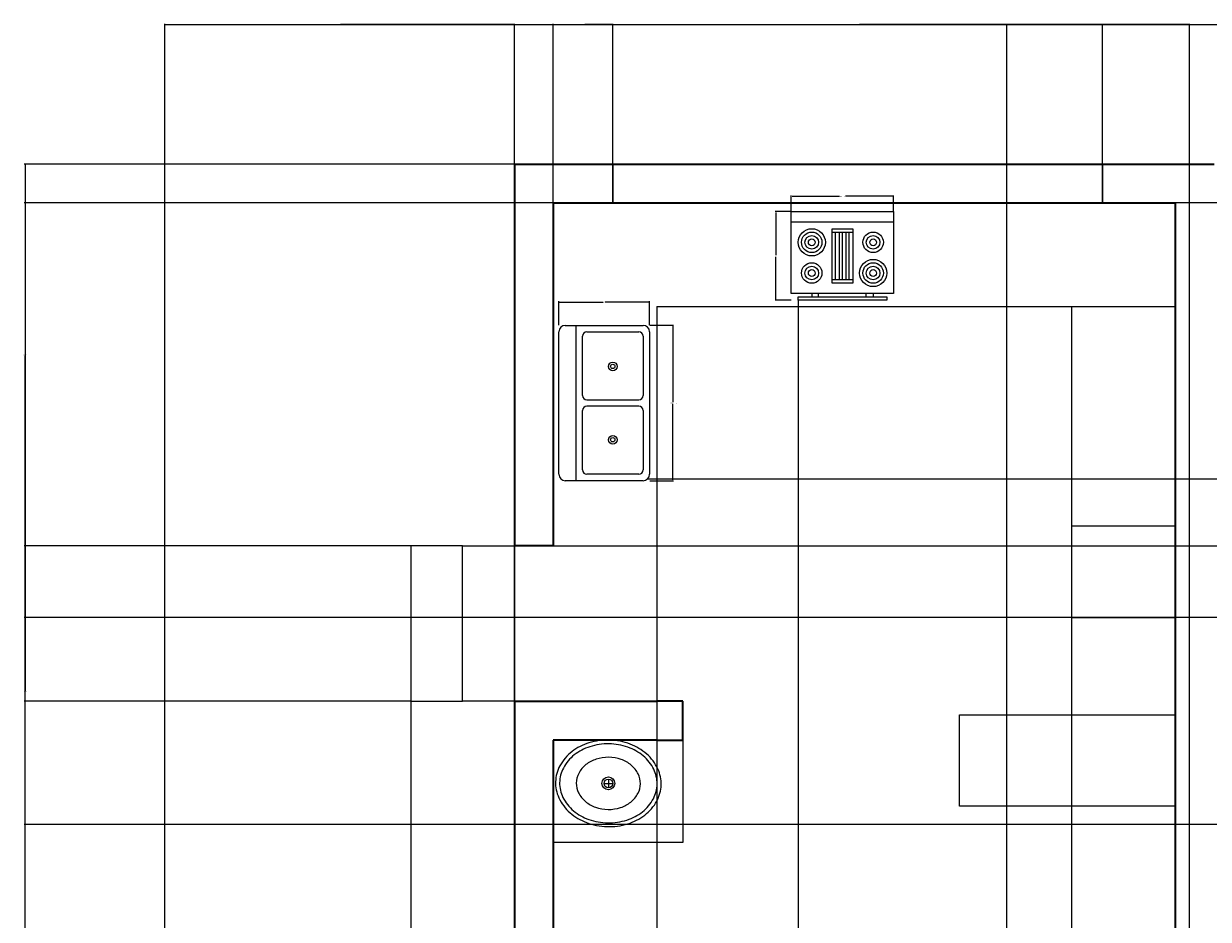
# Model space of a CAD drawing. Units: inches. Extents: x 1159 to 1869, y 2212 to 2738.
# Tile 2 of 5: x 1159 to 1433, y 2531 to 2738. Entities that reach past the tile are written whole.
import ezdxf

# ---------------------------------------------------------------- set-up
doc = ezdxf.new("R2010")
doc.units = ezdxf.units.IN
for name, color, linetype, lineweight in [('A-ANNO-DIMS', 2, 'Continuous', 18), ('A-EQPM', 8, 'Continuous', 18), ('A-FLOR-CASE', 30, 'Continuous', 18), ('A-FLOR-FIXT', 9, 'Continuous', 18), ('A-FLOR-STRS', 7, 'Continuous', 25), ('A-GLAZ', 4, 'Continuous', 18), ('A-WALL', 7, 'Continuous', 35)]:
    doc.layers.add(name, color=color, linetype=linetype, lineweight=lineweight)
doc.styles.get("Standard").update_dxf_attribs({"font": 'arial.ttf'})
doc.dimstyles.get("Standard").update_dxf_attribs({"dimtxt": 0.18, "dimasz": 0.18, "dimexe": 0.18, "dimexo": 0.0625, "dimgap": 0.09, "dimtad": 0, "dimtih": 1, "dimtoh": 1, "dimdec": 4, "dimzin": 0, "dimdsep": 46, "dimtxsty": 'Standard', "dimcen": 0.09, "dimadec": 0, "dimazin": 0, "dimtfac": 1, "dimtdec": 4, "dimtofl": 0, "dimtmove": 0, "dimatfit": 3, "dimfxl": 1, "dimtolj": 1, "dimtzin": 0, "dimarcsym": 0})

# ---------------------------------------------------------------- blocks, each defined once
blk = doc.blocks.new('Sink - Oval top')
for p, q in [((-1, 0), (1, 0)), ((0, 1), (0, -1))]:
    blk.add_line(p, q)
for points in [[(-12.23, 0.39, 0.117634), (-11.46, -3.36, 0.104469), (-8.88, -6.8, 0.090016), (-5.08, -9.07, 0.08192), (-0.32, -10.02, 0.08192), (4.49, -9.38, 0.090016), (8.42, -7.36, 0.104469), (11.22, -4.09, 0.117634), (12.23, -0.39, 0.117634), (11.46, 3.36, 0.104469), (8.88, 6.8, 0.090016), (5.08, 9.07, 0.08192), (0.32, 10.02, 0.08192), (-4.49, 9.38, 0.090016), (-8.42, 7.36, 0.104469), (-11.22, 4.09, 0.117634)], [(-11.29, 0.16, 0.118622), (-10.52, -3.25, 0.104678), (-8.07, -6.36, 0.089562), (-4.54, -8.37, 0.081185), (-0.13, -9.15, 0.081185), (4.3, -8.49, 0.089562), (7.89, -6.58, 0.104678), (10.42, -3.55, 0.118622), (11.29, -0.16, 0.118622), (10.52, 3.25, 0.104678), (8.07, 6.36, 0.089562), (4.54, 8.37, 0.081185), (0.13, 9.15, 0.081185), (-4.3, 8.49, 0.089562), (-7.89, 6.58, 0.104678), (-10.42, 3.55, 0.118622)], [(-7.42, 0.08, 0.118283), (-6.91, -2.17, 0.104607), (-5.29, -4.21, 0.089718), (-2.97, -5.53, 0.081436), (-0.07, -6.04, 0.081436), (2.84, -5.59, 0.089718), (5.2, -4.33, 0.104607), (6.86, -2.32, 0.118283), (7.42, -0.08, 0.118283), (6.91, 2.17, 0.104607), (5.29, 4.21, 0.089718), (2.97, 5.53, 0.081436), (0.07, 6.04, 0.081436), (-2.84, 5.59, 0.089718), (-5.2, 4.33, 0.104607), (-6.86, 2.32, 0.118283)]]:
    blk.add_lwpolyline(points, format="xyb", close=True)
for radius in [1.5, 1]:
    blk.add_circle((0, 0), radius)
blk = doc.blocks.new('Sink-double - 36 in top')
for p, q in [((-18, -4), (18, -4)), ((-0.75, -18.5), (-0.75, -6.5)), ((0.75, -6.5), (0.75, -18.5))]:
    blk.add_line(p, q)
for points in [[(-16.5, 0), (16.5, 0)], [(-18, -19.5), (-18, -1.5)], [(18, -1.5), (18, -19.5)], [(-16.5, -18.5), (-16.5, -6.5)], [(-15.5, -5.5), (-1.75, -5.5)], [(1.75, -5.5), (15.5, -5.5)], [(16.5, -6.5), (16.5, -18.5)], [(16.5, -21), (-16.5, -21)], [(-1.75, -19.5), (-15.5, -19.5)], [(15.5, -19.5), (1.75, -19.5)]]:
    blk.add_lwpolyline(points)
for centre, radius in [((-8.5, -12.5), 1), ((-8.5, -12.5), 0.5), ((8.5, -12.5), 1), ((8.5, -12.5), 0.5)]:
    blk.add_circle(centre, radius)
for centre, radius, start, end in [((-16.5, -1.5), 1.5, 90, 180), ((16.5, -1.5), 1.5, 0, 90), ((-15.5, -6.5), 1, 90, 180), ((-1.75, -6.5), 1, 0, 90), ((1.75, -6.5), 1, 90, 180), ((15.5, -6.5), 1, 0, 90), ((-15.5, -18.5), 1, 180, 270), ((-1.75, -18.5), 1, 270, 0), ((1.75, -18.5), 1, 180, 270), ((15.5, -18.5), 1, 270, 0), ((-16.5, -19.5), 1.5, 180, 270), ((16.5, -19.5), 1.5, 270, 0)]:
    blk.add_arc(centre, radius, start, end)
blk = doc.blocks.new('Range-Oven - 30 in top')
for p, q in [((0, -3), (30, -3)), ((12, -6), (18, -6)), ((13, -20), (13, -6)), ((14, -6), (14, -20)), ((15, -20), (15, -6)), ((16, -6), (16, -20)), ((17, -20), (17, -6)), ((18, -20), (12, -20)), ((6, -24), (6, -25)), ((8, -25), (8, -24)), ((22, -25), (22, -24)), ((24, -24), (24, -25))]:
    blk.add_line(p, q)
for points in [[(0, -24), (0, 0), (30, 0), (30, -24)], [(12, -21), (12, -5), (18, -5), (18, -21)], [(2, -26), (2, -25), (28, -25), (28, -26)]]:
    blk.add_lwpolyline(points, close=True)
for centre, radius in [((6, -9), 4), ((6, -9), 3), ((24, -9), 3), ((6, -9), 2), ((6, -9), 1), ((24, -9), 2), ((24, -9), 1), ((6, -18), 3), ((6, -18), 2), ((6, -18), 1), ((24, -18), 4), ((24, -18), 3), ((24, -18), 2), ((24, -18), 1)]:
    blk.add_circle(centre, radius)
blk = doc.blocks.new('*D16')
at = {"layer": 'A-ANNO-DIMS', "color": 0, "lineweight": -2, "transparency": 16777216}
for p, q in [((1303.74, 2668.28), (1309.26, 2668.28)), ((1309.08, 2668.1), (1309.08, 2650.46)), ((1309.08, 2632.46), (1309.08, 2650.09)), ((1303.74, 2632.28), (1309.26, 2632.28))]:
    blk.add_line(p, q, dxfattribs=at)
at = {"layer": 'A-ANNO-DIMS', "color": 0, "transparency": 16777216}
for points in [[(1309.05, 2668.1), (1309.11, 2668.1), (1309.08, 2668.28)], [(1309.05, 2632.46), (1309.11, 2632.46), (1309.08, 2632.28)]]:
    blk.add_solid(points, dxfattribs=at)
at = {"layer": 'Defpoints', "color": 0, "transparency": 16777216}
for p in [(1303.68, 2668.28), (1309.08, 2668.28), (1303.68, 2632.28)]:
    blk.add_point(p, dxfattribs=at)
at = {"layer": 'A-ANNO-DIMS', "color": 0, "transparency": 16777216, "insert": (1309.08, 2650.28), "char_height": 0.18, "attachment_point": 5}
blk.add_mtext('\\A1;DOUBLE SINK 36', dxfattribs=at)
blk = doc.blocks.new('*D17')
at = {"layer": 'A-ANNO-DIMS', "color": 0, "lineweight": -2, "transparency": 16777216}
for p, q in [((1282.68, 2668.34), (1282.68, 2673.86)), ((1282.86, 2673.68), (1292.97, 2673.68)), ((1303.5, 2673.68), (1293.38, 2673.68)), ((1303.68, 2668.34), (1303.68, 2673.86))]:
    blk.add_line(p, q, dxfattribs=at)
at = {"layer": 'A-ANNO-DIMS', "color": 0, "transparency": 16777216}
for points in [[(1282.86, 2673.71), (1282.86, 2673.65), (1282.68, 2673.68)], [(1303.5, 2673.71), (1303.5, 2673.65), (1303.68, 2673.68)]]:
    blk.add_solid(points, dxfattribs=at)
at = {"layer": 'Defpoints', "color": 0, "transparency": 16777216}
for p in [(1282.68, 2673.68), (1282.68, 2668.28), (1303.68, 2668.28)]:
    blk.add_point(p, dxfattribs=at)
at = {"layer": 'A-ANNO-DIMS', "color": 0, "transparency": 16777216, "insert": (1293.18, 2673.68), "char_height": 0.18, "attachment_point": 5}
blk.add_mtext('\\A1;21', dxfattribs=at)
blk = doc.blocks.new('*D18')
at = {"layer": 'A-ANNO-DIMS', "color": 0, "lineweight": -2, "transparency": 16777216}
for p, q in [((1336.51, 2694.68), (1336.51, 2698.35)), ((1336.69, 2698.17), (1347.66, 2698.17)), ((1360.02, 2698.17), (1349.05, 2698.17)), ((1360.2, 2694.68), (1360.2, 2698.35))]:
    blk.add_line(p, q, dxfattribs=at)
at = {"layer": 'A-ANNO-DIMS', "color": 0, "transparency": 16777216}
for points in [[(1336.69, 2698.2), (1336.69, 2698.14), (1336.51, 2698.17)], [(1360.02, 2698.2), (1360.02, 2698.14), (1360.2, 2698.17)]]:
    blk.add_solid(points, dxfattribs=at)
at = {"layer": 'Defpoints', "color": 0, "transparency": 16777216}
for p in [(1360.2, 2698.17), (1336.51, 2694.61), (1360.2, 2694.61)]:
    blk.add_point(p, dxfattribs=at)
at = {"layer": 'A-ANNO-DIMS', "color": 0, "transparency": 16777216, "insert": (1348.35, 2698.17), "char_height": 0.18, "attachment_point": 5}
blk.add_mtext('\\A1;RANGE 24', dxfattribs=at)
blk = doc.blocks.new('*D19')
at = {"layer": 'A-ANNO-DIMS', "color": 0, "lineweight": -2, "transparency": 16777216}
for p, q in [((1336.44, 2694.61), (1332.77, 2694.61)), ((1332.95, 2694.43), (1332.95, 2684.53)), ((1332.95, 2674.26), (1332.95, 2684.17)), ((1336.44, 2674.08), (1332.77, 2674.08))]:
    blk.add_line(p, q, dxfattribs=at)
at = {"layer": 'A-ANNO-DIMS', "color": 0, "transparency": 16777216}
for points in [[(1332.92, 2694.43), (1332.98, 2694.43), (1332.95, 2694.61)], [(1332.92, 2674.26), (1332.98, 2674.26), (1332.95, 2674.08)]]:
    blk.add_solid(points, dxfattribs=at)
at = {"layer": 'Defpoints', "color": 0, "transparency": 16777216}
for p in [(1332.95, 2694.61), (1336.51, 2694.61), (1336.51, 2674.08)]:
    blk.add_point(p, dxfattribs=at)
at = {"layer": 'A-ANNO-DIMS', "color": 0, "transparency": 16777216, "insert": (1332.95, 2684.35), "char_height": 0.18, "attachment_point": 5}
blk.add_mtext('\\A1;21', dxfattribs=at)
blk = doc.blocks.new('*D20')
at = {"layer": 'A-ANNO-DIMS', "color": 0, "lineweight": -2, "transparency": 16777216}
for p, q in [((1191.4, 2461.27), (1191.4, 2738.15)), ((1191.58, 2737.97), (1513.61, 2737.97)), ((1836.22, 2737.97), (1514.19, 2737.97)), ((1836.4, 2705.69), (1836.4, 2738.15))]:
    blk.add_line(p, q, dxfattribs=at)
at = {"layer": 'A-ANNO-DIMS', "color": 0, "transparency": 16777216}
for points in [[(1191.58, 2738), (1191.58, 2737.94), (1191.4, 2737.97)], [(1836.22, 2738), (1836.22, 2737.94), (1836.4, 2737.97)]]:
    blk.add_solid(points, dxfattribs=at)
at = {"layer": 'Defpoints', "color": 0, "transparency": 16777216}
for p in [(1836.4, 2737.97), (1836.4, 2705.63), (1191.4, 2461.21)]:
    blk.add_point(p, dxfattribs=at)
at = {"layer": 'A-ANNO-DIMS', "color": 0, "transparency": 16777216, "insert": (1513.9, 2737.97), "char_height": 0.18, "attachment_point": 5}
blk.add_mtext('\\A1;645', dxfattribs=at)
blk = doc.blocks.new('*D22')
at = {"layer": 'A-ANNO-DIMS', "color": 0, "lineweight": -2, "transparency": 16777216}
for p, q in [((1191.4, 2461.27), (1191.4, 2738.15)), ((1191.58, 2737.97), (1231.7, 2737.97)), ((1272.22, 2737.97), (1232.1, 2737.97)), ((1272.4, 2461.27), (1272.4, 2738.15))]:
    blk.add_line(p, q, dxfattribs=at)
at = {"layer": 'A-ANNO-DIMS', "color": 0, "transparency": 16777216}
for points in [[(1191.58, 2738), (1191.58, 2737.94), (1191.4, 2737.97)], [(1272.22, 2738), (1272.22, 2737.94), (1272.4, 2737.97)]]:
    blk.add_solid(points, dxfattribs=at)
at = {"layer": 'Defpoints', "color": 0, "transparency": 16777216}
for p in [(1272.4, 2737.97), (1191.4, 2461.21), (1272.4, 2461.21)]:
    blk.add_point(p, dxfattribs=at)
at = {"layer": 'A-ANNO-DIMS', "color": 0, "transparency": 16777216, "insert": (1231.9, 2737.97), "char_height": 0.18, "attachment_point": 5}
blk.add_mtext('\\A1;81', dxfattribs=at)
blk = doc.blocks.new('*D23')
at = {"layer": 'A-ANNO-DIMS', "color": 0, "lineweight": -2, "transparency": 16777216}
for p, q in [((1425.4, 2556.85), (1425.4, 2211.56)), ((1281.4, 2548.45), (1281.4, 2211.56)), ((1281.58, 2211.74), (1353.12, 2211.74)), ((1425.22, 2211.74), (1353.68, 2211.74))]:
    blk.add_line(p, q, dxfattribs=at)
at = {"layer": 'A-ANNO-DIMS', "color": 0, "transparency": 16777216}
for points in [[(1281.58, 2211.77), (1281.58, 2211.71), (1281.4, 2211.74)], [(1425.22, 2211.77), (1425.22, 2211.71), (1425.4, 2211.74)]]:
    blk.add_solid(points, dxfattribs=at)
at = {"layer": 'Defpoints', "color": 0, "transparency": 16777216}
for p in [(1425.4, 2556.91), (1281.4, 2548.52), (1425.4, 2211.74)]:
    blk.add_point(p, dxfattribs=at)
at = {"layer": 'A-ANNO-DIMS', "color": 0, "transparency": 16777216, "insert": (1353.4, 2211.74), "char_height": 0.18, "attachment_point": 5}
blk.add_mtext('\\A1;144', dxfattribs=at)
blk = doc.blocks.new('*D30')
at = {"layer": 'A-ANNO-DIMS', "color": 0, "lineweight": -2, "transparency": 16777216}
for p, q in [((1272.34, 2705.63), (1158.88, 2705.63)), ((1159.06, 2705.45), (1159.06, 2583.6)), ((1159.06, 2461.39), (1159.06, 2583.24)), ((1191.34, 2461.21), (1158.88, 2461.21))]:
    blk.add_line(p, q, dxfattribs=at)
at = {"layer": 'A-ANNO-DIMS', "color": 0, "transparency": 16777216}
for points in [[(1159.03, 2705.45), (1159.09, 2705.45), (1159.06, 2705.63)], [(1159.03, 2461.39), (1159.09, 2461.39), (1159.06, 2461.21)]]:
    blk.add_solid(points, dxfattribs=at)
at = {"layer": 'Defpoints', "color": 0, "transparency": 16777216}
for p in [(1159.06, 2705.63), (1272.4, 2705.63), (1191.4, 2461.21)]:
    blk.add_point(p, dxfattribs=at)
at = {"layer": 'A-ANNO-DIMS', "color": 0, "transparency": 16777216, "insert": (1159.06, 2583.42), "char_height": 0.18, "attachment_point": 5}
blk.add_mtext('\\A1;244.4', dxfattribs=at)
blk = doc.blocks.new('*D40')
at = {"layer": 'A-ANNO-DIMS', "color": 0, "lineweight": -2, "transparency": 16777216}
for p, q in [((1677.34, 2696.63), (1158.88, 2696.63)), ((1159.06, 2696.45), (1159.06, 2648.81)), ((1159.06, 2600.81), (1159.06, 2648.45)), ((1677.34, 2600.63), (1158.88, 2600.63))]:
    blk.add_line(p, q, dxfattribs=at)
at = {"layer": 'A-ANNO-DIMS', "color": 0, "transparency": 16777216}
for points in [[(1159.03, 2696.45), (1159.09, 2696.45), (1159.06, 2696.63)], [(1159.03, 2600.81), (1159.09, 2600.81), (1159.06, 2600.63)]]:
    blk.add_solid(points, dxfattribs=at)
at = {"layer": 'Defpoints', "color": 0, "transparency": 16777216}
for p in [(1159.06, 2696.63), (1677.4, 2696.63), (1677.4, 2600.63)]:
    blk.add_point(p, dxfattribs=at)
at = {"layer": 'A-ANNO-DIMS', "color": 0, "transparency": 16777216, "insert": (1159.06, 2648.63), "char_height": 0.18, "attachment_point": 5}
blk.add_mtext('\\A1;96', dxfattribs=at)
blk = doc.blocks.new('*D49')
at = {"layer": 'A-ANNO-DIMS', "color": 0, "lineweight": -2, "transparency": 16777216}
for p, q in [((1248.4, 2581.14), (1248.4, 2211.56)), ((1272.4, 2581.14), (1272.4, 2211.56)), ((1248.58, 2211.74), (1260.18, 2211.74)), ((1272.22, 2211.74), (1260.62, 2211.74))]:
    blk.add_line(p, q, dxfattribs=at)
at = {"layer": 'A-ANNO-DIMS', "color": 0, "transparency": 16777216}
for points in [[(1248.58, 2211.77), (1248.58, 2211.71), (1248.4, 2211.74)], [(1272.22, 2211.77), (1272.22, 2211.71), (1272.4, 2211.74)]]:
    blk.add_solid(points, dxfattribs=at)
at = {"layer": 'Defpoints', "color": 0, "transparency": 16777216}
for p in [(1248.4, 2581.21), (1272.4, 2581.21), (1272.4, 2211.74)]:
    blk.add_point(p, dxfattribs=at)
at = {"layer": 'A-ANNO-DIMS', "color": 0, "transparency": 16777216, "insert": (1260.4, 2211.74), "char_height": 0.18, "attachment_point": 5}
blk.add_mtext('\\A1;24', dxfattribs=at)
blk = doc.blocks.new('*D50')
at = {"layer": 'A-ANNO-DIMS', "color": 0, "lineweight": -2, "transparency": 16777216}
for p, q in [((1248.34, 2617.21), (1158.88, 2617.21)), ((1159.06, 2617.03), (1159.06, 2599.39)), ((1159.06, 2581.39), (1159.06, 2599.02)), ((1248.34, 2581.21), (1158.88, 2581.21))]:
    blk.add_line(p, q, dxfattribs=at)
at = {"layer": 'A-ANNO-DIMS', "color": 0, "transparency": 16777216}
for points in [[(1159.03, 2617.03), (1159.09, 2617.03), (1159.06, 2617.21)], [(1159.03, 2581.39), (1159.09, 2581.39), (1159.06, 2581.21)]]:
    blk.add_solid(points, dxfattribs=at)
at = {"layer": 'Defpoints', "color": 0, "transparency": 16777216}
for p in [(1159.06, 2617.21), (1248.4, 2617.21), (1248.4, 2581.21)]:
    blk.add_point(p, dxfattribs=at)
at = {"layer": 'A-ANNO-DIMS', "color": 0, "transparency": 16777216, "insert": (1159.06, 2599.21), "char_height": 0.18, "attachment_point": 5}
blk.add_mtext('\\A1;36', dxfattribs=at)
blk = doc.blocks.new('*D51')
at = {"layer": 'A-ANNO-DIMS', "color": 0, "lineweight": -2, "transparency": 16777216}
for p, q in [((1272.34, 2705.63), (1158.88, 2705.63)), ((1159.06, 2705.45), (1159.06, 2661.6)), ((1159.06, 2617.39), (1159.06, 2661.24)), ((1248.34, 2617.21), (1158.88, 2617.21))]:
    blk.add_line(p, q, dxfattribs=at)
at = {"layer": 'A-ANNO-DIMS', "color": 0, "transparency": 16777216}
for points in [[(1159.03, 2705.45), (1159.09, 2705.45), (1159.06, 2705.63)], [(1159.03, 2617.39), (1159.09, 2617.39), (1159.06, 2617.21)]]:
    blk.add_solid(points, dxfattribs=at)
at = {"layer": 'Defpoints', "color": 0, "transparency": 16777216}
for p in [(1159.06, 2705.63), (1272.4, 2705.63), (1248.4, 2617.21)]:
    blk.add_point(p, dxfattribs=at)
at = {"layer": 'A-ANNO-DIMS', "color": 0, "transparency": 16777216, "insert": (1159.06, 2661.42), "char_height": 0.18, "attachment_point": 5}
blk.add_mtext('\\A1;88.42', dxfattribs=at)
blk = doc.blocks.new('*D52')
at = {"layer": 'A-ANNO-DIMS', "color": 0, "lineweight": -2, "transparency": 16777216}
for p, q in [((1386.4, 2452.27), (1386.4, 2738.15)), ((1386.58, 2737.97), (1407.18, 2737.97)), ((1428.56, 2737.97), (1407.97, 2737.97)), ((1428.74, 2458.27), (1428.74, 2738.15))]:
    blk.add_line(p, q, dxfattribs=at)
at = {"layer": 'A-ANNO-DIMS', "color": 0, "transparency": 16777216}
for points in [[(1386.58, 2738), (1386.58, 2737.94), (1386.4, 2737.97)], [(1428.56, 2738), (1428.56, 2737.94), (1428.74, 2737.97)]]:
    blk.add_solid(points, dxfattribs=at)
at = {"layer": 'Defpoints', "color": 0, "transparency": 16777216}
for p in [(1428.74, 2737.97), (1428.74, 2458.21), (1386.4, 2452.21)]:
    blk.add_point(p, dxfattribs=at)
at = {"layer": 'A-ANNO-DIMS', "color": 0, "transparency": 16777216, "insert": (1407.57, 2737.97), "char_height": 0.18, "attachment_point": 5}
blk.add_mtext('\\A1;42.34', dxfattribs=at)
blk = doc.blocks.new('*D59')
at = {"layer": 'A-ANNO-DIMS', "color": 0, "lineweight": -2, "transparency": 16777216}
for p, q in [((1401.4, 2600.57), (1401.4, 2211.56)), ((1425.4, 2600.57), (1425.4, 2211.56)), ((1401.58, 2211.74), (1413.18, 2211.74)), ((1425.22, 2211.74), (1413.62, 2211.74))]:
    blk.add_line(p, q, dxfattribs=at)
at = {"layer": 'A-ANNO-DIMS', "color": 0, "transparency": 16777216}
for points in [[(1401.58, 2211.77), (1401.58, 2211.71), (1401.4, 2211.74)], [(1425.22, 2211.77), (1425.22, 2211.71), (1425.4, 2211.74)]]:
    blk.add_solid(points, dxfattribs=at)
at = {"layer": 'Defpoints', "color": 0, "transparency": 16777216}
for p in [(1401.4, 2600.63), (1425.4, 2600.63), (1425.4, 2211.74)]:
    blk.add_point(p, dxfattribs=at)
at = {"layer": 'A-ANNO-DIMS', "color": 0, "transparency": 16777216, "insert": (1413.4, 2211.74), "char_height": 0.18, "attachment_point": 5}
blk.add_mtext('\\A1;24', dxfattribs=at)
blk = doc.blocks.new('*D62')
at = {"layer": 'A-ANNO-DIMS', "color": 0, "lineweight": -2, "transparency": 16777216}
for p, q in [((1281.4, 2696.69), (1281.4, 2738.15)), ((1281.58, 2737.97), (1287.82, 2737.97)), ((1294.98, 2737.97), (1288.73, 2737.97)), ((1295.16, 2696.69), (1295.16, 2738.15))]:
    blk.add_line(p, q, dxfattribs=at)
at = {"layer": 'A-ANNO-DIMS', "color": 0, "transparency": 16777216}
for points in [[(1281.58, 2738), (1281.58, 2737.94), (1281.4, 2737.97)], [(1294.98, 2738), (1294.98, 2737.94), (1295.16, 2737.97)]]:
    blk.add_solid(points, dxfattribs=at)
at = {"layer": 'Defpoints', "color": 0, "transparency": 16777216}
for p in [(1295.16, 2737.97), (1281.4, 2696.63), (1295.16, 2696.63)]:
    blk.add_point(p, dxfattribs=at)
at = {"layer": 'A-ANNO-DIMS', "color": 0, "transparency": 16777216, "insert": (1288.28, 2737.97), "char_height": 0.18, "attachment_point": 5}
blk.add_mtext('\\A1;13.756', dxfattribs=at)
blk = doc.blocks.new('*D63')
at = {"layer": 'A-ANNO-DIMS', "color": 0, "lineweight": -2, "transparency": 16777216}
for p, q in [((1295.16, 2696.69), (1295.16, 2738.15)), ((1295.34, 2737.97), (1351.41, 2737.97)), ((1408.4, 2737.97), (1352.32, 2737.97)), ((1408.58, 2696.69), (1408.58, 2738.15))]:
    blk.add_line(p, q, dxfattribs=at)
at = {"layer": 'A-ANNO-DIMS', "color": 0, "transparency": 16777216}
for points in [[(1295.34, 2738), (1295.34, 2737.94), (1295.16, 2737.97)], [(1408.4, 2738), (1408.4, 2737.94), (1408.58, 2737.97)]]:
    blk.add_solid(points, dxfattribs=at)
at = {"layer": 'Defpoints', "color": 0, "transparency": 16777216}
for p in [(1408.58, 2737.97), (1295.16, 2696.63), (1408.58, 2696.63)]:
    blk.add_point(p, dxfattribs=at)
at = {"layer": 'A-ANNO-DIMS', "color": 0, "transparency": 16777216, "insert": (1351.87, 2737.97), "char_height": 0.18, "attachment_point": 5}
blk.add_mtext('\\A1;113.42', dxfattribs=at)
blk = doc.blocks.new('*D69')
at = {"layer": 'A-ANNO-DIMS', "color": 0, "lineweight": -2, "transparency": 16777216}
for p, q in [((1803.34, 2696.63), (1158.88, 2696.63)), ((1159.06, 2696.45), (1159.06, 2624.81)), ((1159.06, 2552.81), (1159.06, 2624.45)), ((1803.34, 2552.63), (1158.88, 2552.63))]:
    blk.add_line(p, q, dxfattribs=at)
at = {"layer": 'A-ANNO-DIMS', "color": 0, "transparency": 16777216}
for points in [[(1159.03, 2696.45), (1159.09, 2696.45), (1159.06, 2696.63)], [(1159.03, 2552.81), (1159.09, 2552.81), (1159.06, 2552.63)]]:
    blk.add_solid(points, dxfattribs=at)
at = {"layer": 'Defpoints', "color": 0, "transparency": 16777216}
for p in [(1159.06, 2696.63), (1803.4, 2696.63), (1803.4, 2552.63)]:
    blk.add_point(p, dxfattribs=at)
at = {"layer": 'A-ANNO-DIMS', "color": 0, "transparency": 16777216, "insert": (1159.06, 2624.63), "char_height": 0.18, "attachment_point": 5}
blk.add_mtext('\\A1;144', dxfattribs=at)
blk = doc.blocks.new('*D72')
at = {"layer": 'A-ANNO-DIMS', "color": 0, "lineweight": -2, "transparency": 16777216}
for p, q in [((1305.4, 2672.57), (1305.4, 2211.56)), ((1338.09, 2674.02), (1338.09, 2211.56)), ((1305.58, 2211.74), (1321.28, 2211.74)), ((1337.91, 2211.74), (1322.21, 2211.74))]:
    blk.add_line(p, q, dxfattribs=at)
at = {"layer": 'A-ANNO-DIMS', "color": 0, "transparency": 16777216}
for points in [[(1305.58, 2211.77), (1305.58, 2211.71), (1305.4, 2211.74)], [(1337.91, 2211.77), (1337.91, 2211.71), (1338.09, 2211.74)]]:
    blk.add_solid(points, dxfattribs=at)
at = {"layer": 'Defpoints', "color": 0, "transparency": 16777216}
for p in [(1305.4, 2672.63), (1338.09, 2674.08), (1338.09, 2211.74)]:
    blk.add_point(p, dxfattribs=at)
at = {"layer": 'A-ANNO-DIMS', "color": 0, "transparency": 16777216, "insert": (1321.74, 2211.74), "char_height": 0.18, "attachment_point": 5}
blk.add_mtext('\\A1;32.685', dxfattribs=at)
blk = doc.blocks.new('*D73')
at = {"layer": 'A-ANNO-DIMS', "color": 0, "lineweight": -2, "transparency": 16777216}
for p, q in [((1303.3, 2632.72), (1868.92, 2632.72)), ((1868.74, 2632.54), (1868.74, 2625.14)), ((1868.74, 2617.39), (1868.74, 2624.78)), ((1305.46, 2617.21), (1868.92, 2617.21))]:
    blk.add_line(p, q, dxfattribs=at)
at = {"layer": 'A-ANNO-DIMS', "color": 0, "transparency": 16777216}
for points in [[(1868.71, 2632.54), (1868.77, 2632.54), (1868.74, 2632.72)], [(1868.71, 2617.39), (1868.77, 2617.39), (1868.74, 2617.21)]]:
    blk.add_solid(points, dxfattribs=at)
at = {"layer": 'Defpoints', "color": 0, "transparency": 16777216}
for p in [(1303.24, 2632.72), (1868.74, 2632.72), (1305.4, 2617.21)]:
    blk.add_point(p, dxfattribs=at)
at = {"layer": 'A-ANNO-DIMS', "color": 0, "transparency": 16777216, "insert": (1868.74, 2624.96), "char_height": 0.18, "attachment_point": 5}
blk.add_mtext('\\A1;15.51', dxfattribs=at)

msp = doc.modelspace()

# ---------------------------------------------------------------- linework, layer by layer
at = {"layer": 'A-FLOR-CASE'}
for p, q in [((1305.4011, 2672.6279), (1305.4011, 2617.2064)), ((1305.4011, 2672.6279), (1425.4011, 2672.6279)), ((1401.4011, 2672.6279), (1401.4011, 2556.9124)), ((1401.4011, 2621.8522), (1425.4011, 2621.8522)), ((1281.4011, 2617.2064), (1305.4011, 2617.2064)), ((1401.4011, 2600.6279), (1425.4011, 2600.6279)), ((1375.4906, 2556.9124), (1375.4906, 2578.0775)), ((1375.4906, 2578.0775), (1401.4011, 2578.0775)), ((1401.4011, 2578.0775), (1425.4011, 2578.0775)), ((1311.4011, 2572.2064), (1311.4011, 2548.5157)), ((1425.4011, 2556.9124), (1375.4906, 2556.9124)), ((1311.4011, 2548.5157), (1281.4011, 2548.5157))]:
    msp.add_line(p, q, dxfattribs=at)
at = {"layer": 'A-FLOR-STRS'}
for p, q in [((1260.4011, 2617.2064), (1248.4011, 2617.2064)), ((1248.4011, 2617.2064), (1248.4011, 2581.2064)), ((1260.4011, 2581.2064), (1260.4011, 2617.2064)), ((1260.4011, 2617.2064), (1272.4011, 2617.2064)), ((1272.4011, 2617.2064), (1272.4011, 2581.2064)), ((1248.4011, 2581.2064), (1260.4011, 2581.2064)), ((1272.4011, 2581.2064), (1260.4011, 2581.2064))]:
    msp.add_line(p, q, dxfattribs=at)
at = {"layer": 'A-GLAZ'}
for p, q in [((1295.1569, 2705.6279), (1295.1569, 2696.6279)), ((1408.5791, 2705.6279), (1408.5791, 2696.6279))]:
    msp.add_line(p, q, dxfattribs=at)
at = {"layer": 'A-WALL'}
for p, q in [((1272.4011, 2705.6279), (1434.4011, 2705.6279)), ((1272.4011, 2705.6279), (1272.4011, 2617.2064)), ((1281.4011, 2696.6279), (1425.4011, 2696.6279)), ((1281.4011, 2696.6279), (1281.4011, 2617.2064)), ((1425.4011, 2696.6279), (1425.4011, 2504.6279)), ((1281.4011, 2617.2064), (1272.4011, 2617.2064)), ((1272.4011, 2581.2064), (1305.4011, 2581.2064)), ((1272.4011, 2581.2064), (1272.4011, 2452.2064)), ((1311.4011, 2581.2064), (1305.4011, 2581.2064)), ((1311.4011, 2572.2064), (1311.4011, 2581.2064)), ((1305.4011, 2572.2064), (1281.4011, 2572.2064)), ((1281.4011, 2572.2064), (1281.4011, 2452.2064)), ((1305.4011, 2572.2064), (1311.4011, 2572.2064))]:
    msp.add_line(p, q, dxfattribs=at)

# ---------------------------------------------------------------- block references
at = {"layer": 'A-EQPM', "xscale": 0.7897525270488926, "yscale": 0.7897525270488926, "zscale": 0.7897525270488926}
msp.add_blockref('Range-Oven - 30 in top', (1336.5062, 2694.6131), dxfattribs=at)
at = {"layer": 'A-FLOR-FIXT', "rotation": 90}
msp.add_blockref('Sink-double - 36 in top', (1282.6771, 2650.278), dxfattribs=at)
at = {"layer": 'A-FLOR-FIXT'}
msp.add_blockref('Sink - Oval top', (1294.1451, 2562.1906), dxfattribs=at)

# ---------------------------------------------------------------- dimensions: what is measured, and where the dimension line sits
at = {"layer": 'A-ANNO-DIMS'}
for base, p1, p2, override, picture, middle in [((1836.4011, 2737.9679), (1191.4011, 2461.2064), (1836.4011, 2705.6279), {"dimdec": 0, "dimlfac": 1, "dimrnd": 0, "dimzin": 0, "dimdsep": 46, "dimlunit": 2}, '*D20', (1513.9011, 2737.9679)), ((1272.4011, 2737.9679), (1191.4011, 2461.2064), (1272.4011, 2461.2064), {"dimdec": 0, "dimlfac": 1, "dimrnd": 0, "dimzin": 0, "dimdsep": 46, "dimlunit": 2}, '*D22', (1231.9011, 2737.9679)), ((1295.1569, 2737.9679), (1281.4011, 2696.6279), (1295.1569, 2696.6279), {"dimdec": 3, "dimlfac": 1, "dimrnd": 0, "dimzin": 0, "dimdsep": 46, "dimlunit": 2}, '*D62', (1288.279, 2737.9679)), ((1408.5791, 2737.9679), (1295.1569, 2696.6279), (1408.5791, 2696.6279), {"dimdec": 2, "dimlfac": 1, "dimrnd": 0, "dimzin": 0, "dimdsep": 46, "dimlunit": 2}, '*D63', (1351.868, 2737.9679)), ((1428.7443, 2737.9679), (1386.4011, 2452.2064), (1428.7443, 2458.2064), {"dimdec": 2, "dimlfac": 1, "dimrnd": 0, "dimzin": 0, "dimdsep": 46, "dimlunit": 2}, '*D52', (1407.5727, 2737.9679)), ((1338.0857, 2211.7357), (1305.4011, 2672.6279), (1338.0857, 2674.0796), {"dimdec": 3, "dimlfac": 1, "dimrnd": 0, "dimzin": 0, "dimdsep": 46, "dimlunit": 2}, '*D72', (1321.7434, 2211.7357)), ((1425.4011, 2211.7357), (1401.4011, 2600.6279), (1425.4011, 2600.6279), {"dimdec": 0, "dimlfac": 1, "dimrnd": 0, "dimzin": 0, "dimdsep": 46, "dimlunit": 2}, '*D59', (1413.4011, 2211.7357)), ((1272.4011, 2211.7357), (1248.4011, 2581.2064), (1272.4011, 2581.2064), {"dimdec": 0, "dimlfac": 1, "dimrnd": 0, "dimzin": 0, "dimdsep": 46, "dimlunit": 2}, '*D49', (1260.4011, 2211.7357)), ((1425.4011, 2211.7357), (1281.4011, 2548.5157), (1425.4011, 2556.9124), {"dimdec": 0, "dimlfac": 1, "dimrnd": 0, "dimzin": 0, "dimdsep": 46, "dimlunit": 2}, '*D23', (1353.4011, 2211.7357))]:
    dim = msp.add_linear_dim(base=base, p1=p1, p2=p2, dimstyle='Standard', override=override, dxfattribs=at)
    dim.commit()
    dim.dimension.update_dxf_attribs({"geometry": picture, "text_midpoint": middle})
for base, p1, p2, angle, override, picture, middle in [((1159.0611, 2705.6279), (1191.4011, 2461.2064), (1272.4011, 2705.6279), 90, {"dimdec": 1, "dimlfac": 1, "dimrnd": 0, "dimzin": 0, "dimdsep": 46, "dimlunit": 2}, '*D30', (1159.0611, 2583.4172)), ((1159.0611, 2705.6279), (1248.4011, 2617.2064), (1272.4011, 2705.6279), 90, {"dimdec": 2, "dimlfac": 1, "dimrnd": 0, "dimzin": 0, "dimdsep": 46, "dimlunit": 2}, '*D51', (1159.0611, 2661.4172)), ((1159.0611, 2696.6279), (1803.4011, 2552.6279), (1803.4011, 2696.6279), 90, {"dimdec": 0, "dimlfac": 1, "dimrnd": 0, "dimzin": 0, "dimdsep": 46, "dimlunit": 2}, '*D69', (1159.0611, 2624.6279)), ((1159.0611, 2696.6279), (1677.4011, 2600.6279), (1677.4011, 2696.6279), 90, {"dimdec": 0, "dimlfac": 1, "dimrnd": 0, "dimzin": 0, "dimdsep": 46, "dimlunit": 2}, '*D40', (1159.0611, 2648.6279)), ((1332.9523, 2694.6131), (1336.5062, 2674.0796), (1336.5062, 2694.6131), 90, {"dimdec": 0, "dimlfac": 1, "dimrnd": 0, "dimzin": 0, "dimdsep": 46, "dimlunit": 2}, '*D19', (1332.9523, 2684.3463)), ((1282.6771, 2673.678), (1303.6771, 2668.278), (1282.6771, 2668.278), 180, {"dimdec": 0, "dimlfac": 1, "dimrnd": 0, "dimzin": 0, "dimdsep": 46, "dimlunit": 2}, '*D17', (1293.1771, 2673.678)), ((1868.7411, 2632.7174), (1305.4011, 2617.2064), (1303.2377, 2632.7174), 90, {"dimdec": 2, "dimlfac": 1, "dimrnd": 0, "dimzin": 0, "dimdsep": 46, "dimlunit": 2}, '*D73', (1868.7411, 2624.9619)), ((1159.0611, 2617.2064), (1248.4011, 2581.2064), (1248.4011, 2617.2064), 90, {"dimdec": 0, "dimlfac": 1, "dimrnd": 0, "dimzin": 0, "dimdsep": 46, "dimlunit": 2}, '*D50', (1159.0611, 2599.2064))]:
    dim = msp.add_linear_dim(base=base, p1=p1, p2=p2, angle=angle, dimstyle='Standard', override=override, dxfattribs=at)
    dim.commit()
    dim.dimension.update_dxf_attribs({"geometry": picture, "text_midpoint": middle})
dim = msp.add_linear_dim(base=(1360.1988, 2698.167), p1=(1336.5062, 2694.6131), p2=(1360.1988, 2694.6131), text='RANGE <>', dimstyle='Standard', override={"dimdec": 0, "dimlfac": 1, "dimrnd": 0, "dimzin": 0, "dimdsep": 46, "dimlunit": 2}, dxfattribs=at)
dim.commit()
dim.dimension.update_dxf_attribs({"geometry": '*D18', "text_midpoint": (1348.3525, 2698.167)})
dim = msp.add_linear_dim(base=(1309.0771, 2668.278), p1=(1303.6771, 2632.278), p2=(1303.6771, 2668.278), angle=90, text='DOUBLE SINK <>', dimstyle='Standard', override={"dimdec": 0, "dimlfac": 1, "dimrnd": 0, "dimzin": 0, "dimdsep": 46, "dimlunit": 2}, dxfattribs=at)
dim.commit()
dim.dimension.update_dxf_attribs({"geometry": '*D16', "text_midpoint": (1309.0771, 2650.278)})

doc.saveas('drawing.dxf')
